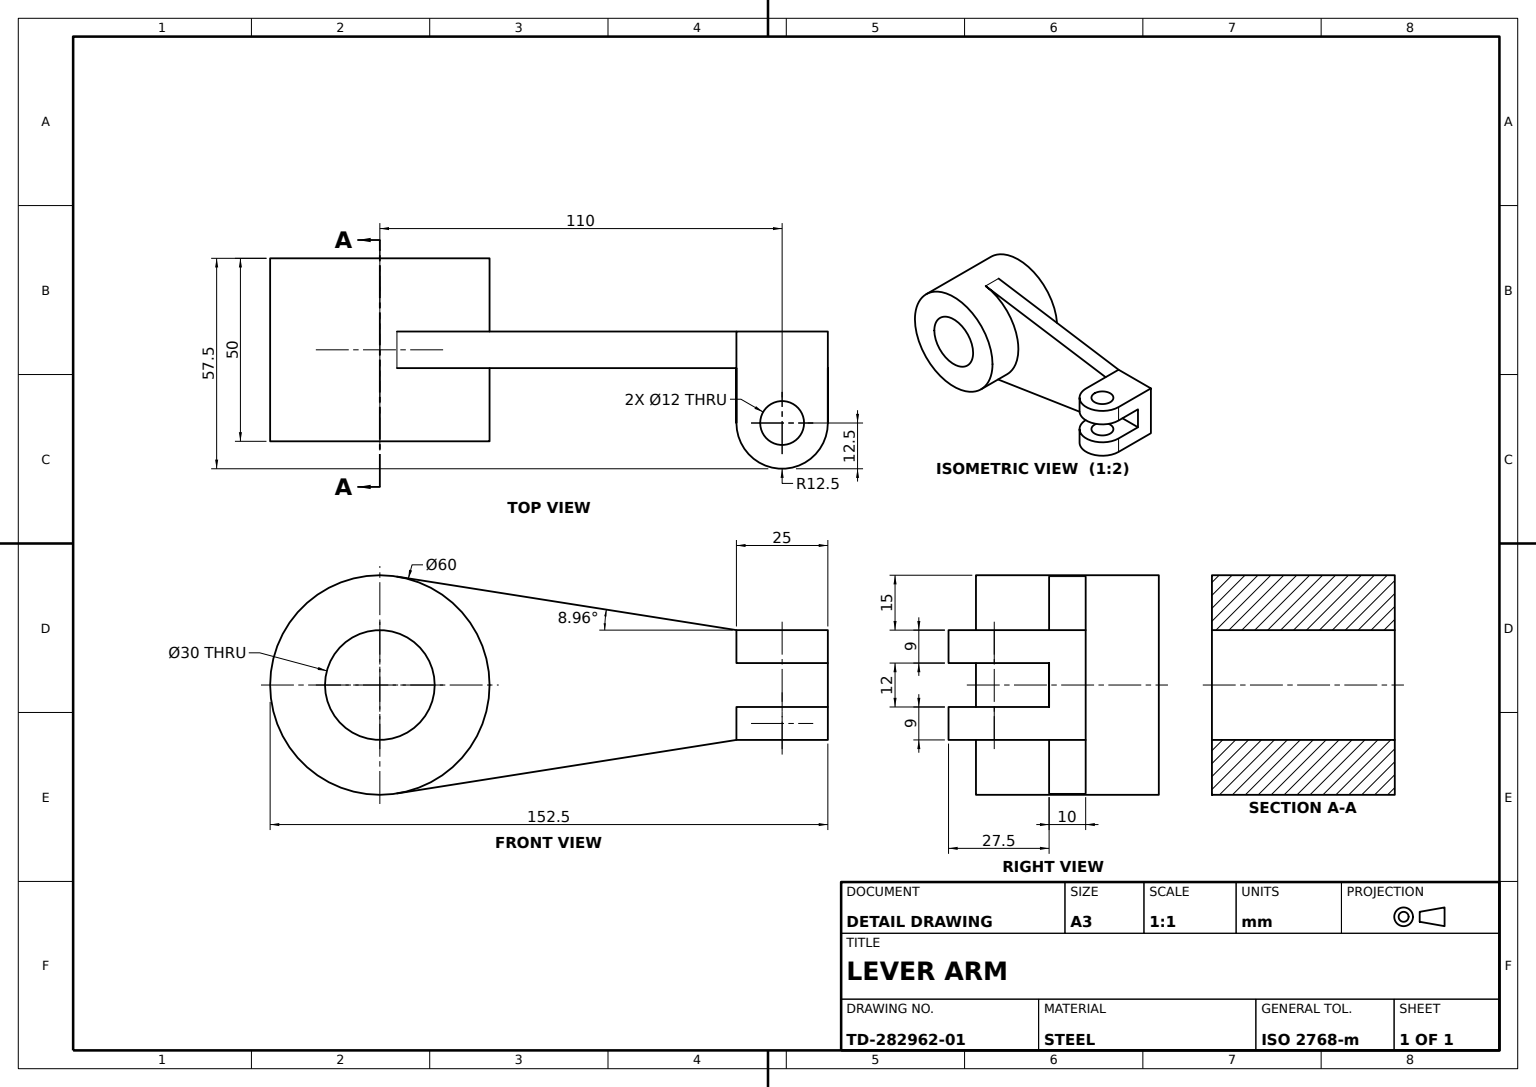
from build123d import *

# Parameters (mm, degrees)
HUB_PROFILE_SKETCH_R   = 30
HUB_PROFILE_SKETCH_R_2 = 15
HUB_60_BORE_30_DEPTH   = 25
LEVER_ARM_WEB_DEPTH    = 5
CLEVIS_LUG_SKETCH_R    = 6
CLEVIS_LUG_DEPTH       = 9


with BuildPart() as part:
    # Hub Profile Sketch → Hub Ø60 Bore Ø30 (new, symmetric)
    with BuildSketch(Plane.XY):
        Circle(HUB_PROFILE_SKETCH_R)
        Circle(HUB_PROFILE_SKETCH_R_2, mode=Mode.SUBTRACT)
    extrude(amount=HUB_60_BORE_30_DEPTH, both=True)

    # Lever Arm Sketch → Lever Arm Web (add, symmetric)
    with BuildSketch(Plane.XY):
        with BuildLine():
            Line((4.671688756, 29.634023084), (97.5, 15))
            Line((97.5, 15), (122.5, 15))
            Line((122.5, 15), (122.5, -15))
            Line((122.5, -15), (97.5, -15))
            Line((97.5, -15), (4.671688756, -29.634023084))
            ThreePointArc((4.671688756, -29.634023084), (30, 0), (4.671688756, 29.634023084))
        make_face()
    extrude(amount=LEVER_ARM_WEB_DEPTH, both=True)

    # Clevis Lug Sketch → Clevis Lug (add)
    with BuildSketch(Plane.XZ.offset(15)):
        with BuildLine():
            Line((97.5, 5), (97.5, 20))
            ThreePointArc((97.5, 20), (110, 32.5), (122.5, 20))
            Line((122.5, 20), (122.5, 5))
            Line((122.5, 5), (97.5, 5))
        make_face()
        with Locations((110, 20)):
            Circle(CLEVIS_LUG_SKETCH_R, mode=Mode.SUBTRACT)
    clevis_lug = extrude(amount=-CLEVIS_LUG_DEPTH)

    # Clevis Lug Mirror: Clevis Lug across plane
    add(clevis_lug.mirror(Plane.ZX))


solid = part.part
